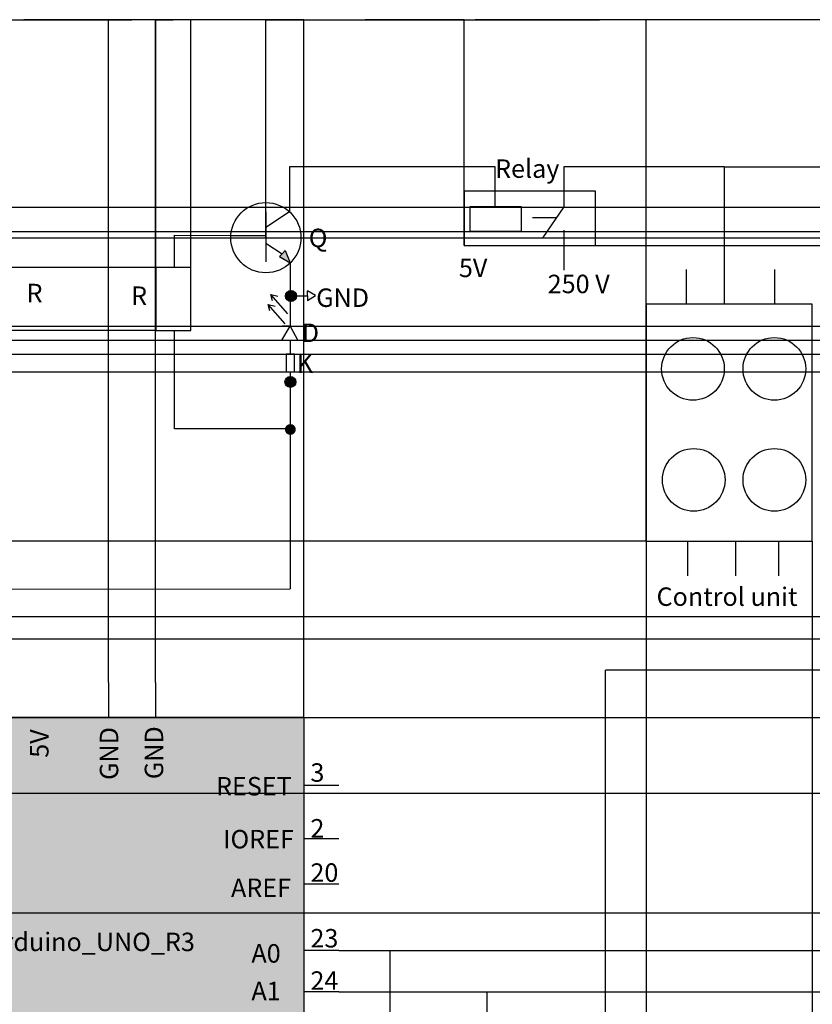
# Model space of a CAD drawing. Units: inches. Extents: x 35362 to 73946, y 43607 to 67532.
# Tile 134 of 134: x 57838 to 67327, y 55752 to 67532. Entities that reach past the tile are written whole.
import ezdxf

# ---------------------------------------------------------------- set-up
doc = ezdxf.new("R2010")
doc.units = ezdxf.units.IN
doc.header["$MEASUREMENT"] = 0
for name, color, linetype, lineweight in [('A-ANNO-DIMS', 2, 'Continuous', 18), ('E-ANNO-TEXT', 5, 'Continuous', 18), ('E-SYMB', 1, 'Continuous', 25), ('E-SYMB-PATT', 1, 'Continuous', 13), ('E-WIRE', 3, 'Continuous', 25)]:
    doc.layers.add(name, color=color, linetype=linetype, lineweight=lineweight)
doc.styles.get("Standard").update_dxf_attribs({"font": 'arial.ttf'})
doc.dimstyles.get("Standard").update_dxf_attribs({"dimtxt": 0.18, "dimasz": 0.18, "dimexe": 0.18, "dimexo": 0.0625, "dimgap": 0.09, "dimtad": 0, "dimtih": 1, "dimtoh": 1, "dimdec": 4, "dimzin": 0, "dimdsep": 46, "dimtxsty": 'Standard', "dimcen": 0.09, "dimadec": 0, "dimazin": 0, "dimtfac": 1, "dimtdec": 4, "dimtofl": 0, "dimtmove": 0, "dimatfit": 3, "dimfxl": 1, "dimtolj": 1, "dimtzin": 0, "dimarcsym": 0})

# ---------------------------------------------------------------- blocks, each defined once
blk = doc.blocks.new('*D8')
at = {"layer": 'A-ANNO-DIMS', "color": 0, "lineweight": -2, "transparency": 16777216}
for p, q in [((66271.28651900003, 65771.51172800003), (73945.82566600003, 65771.51172800003)), ((73945.64566600005, 65771.33172800003), (73945.64566600005, 59737.03093663782)), ((73945.64566600005, 53702.36633900002), (73945.64566600005, 59736.66713036224)), ((72185.70816600003, 53702.18633900003), (73945.82566600003, 53702.18633900003))]:
    blk.add_line(p, q, dxfattribs=at)
at = {"layer": 'A-ANNO-DIMS', "color": 0, "transparency": 16777216}
for points in [[(73945.61566600006, 65771.33172800003), (73945.67566600005, 65771.33172800003), (73945.64566600005, 65771.51172800003)], [(73945.61566600006, 53702.36633900002), (73945.67566600005, 53702.36633900002), (73945.64566600005, 53702.18633900003)]]:
    blk.add_solid(points, dxfattribs=at)
at = {"layer": 'Defpoints', "color": 0, "transparency": 16777216}
for p in [(66271.22401900003, 65771.51172800003), (73945.64566600005, 65771.51172800003), (72185.64566600003, 53702.18633900003)]:
    blk.add_point(p, dxfattribs=at)
at = {"layer": 'A-ANNO-DIMS', "color": 0, "transparency": 16777216, "insert": (73945.64566600005, 59736.84903349999), "char_height": 0.18, "attachment_point": 5}
blk.add_mtext('\\A1;12069', dxfattribs=at)
blk = doc.blocks.new('*D9')
at = {"layer": 'A-ANNO-DIMS', "color": 0, "lineweight": -2, "transparency": 16777216}
for p, q in [((56873.601939, 59185.206457), (56873.601939, 67531.691728)), ((56873.78193899999, 67531.51172799998), (59056.89224322987, 67531.51172799998)), ((61240.727336, 67531.51172799998), (59057.61703177011, 67531.51172799998)), ((61240.907336, 59185.206457), (61240.907336, 67531.691728))]:
    blk.add_line(p, q, dxfattribs=at)
at = {"layer": 'A-ANNO-DIMS', "color": 0, "transparency": 16777216}
for points in [[(56873.78193899999, 67531.541728), (56873.78193899999, 67531.481728), (56873.601939, 67531.51172799998)], [(61240.727336, 67531.541728), (61240.727336, 67531.481728), (61240.907336, 67531.51172799998)]]:
    blk.add_solid(points, dxfattribs=at)
at = {"layer": 'Defpoints', "color": 0, "transparency": 16777216}
for p in [(61240.907336, 67531.51172799998), (56873.601939, 59185.14395699999), (61240.907336, 59185.14395699999)]:
    blk.add_point(p, dxfattribs=at)
at = {"layer": 'A-ANNO-DIMS', "color": 0, "transparency": 16777216, "insert": (59057.25463749999, 67531.51172799998), "char_height": 0.18, "attachment_point": 5}
blk.add_mtext('\\A1;4367', dxfattribs=at)
blk = doc.blocks.new('*D10')
at = {"layer": 'A-ANNO-DIMS', "color": 0, "lineweight": -2, "transparency": 16777216}
for p, q in [((61240.96983600002, 59185.14395700003), (73945.82566600003, 59185.14395700003)), ((73945.64566600005, 59184.96395700003), (73945.64566600005, 56268.51827402935)), ((73945.64566600005, 53351.70866200003), (73945.64566600005, 56268.1543449707)), ((61240.96983600002, 53351.52866200003), (73945.82566600003, 53351.52866200003))]:
    blk.add_line(p, q, dxfattribs=at)
at = {"layer": 'A-ANNO-DIMS', "color": 0, "transparency": 16777216}
for points in [[(73945.61566600006, 59184.96395700003), (73945.67566600005, 59184.96395700003), (73945.64566600005, 59185.14395700003)], [(73945.61566600006, 53351.70866200003), (73945.67566600005, 53351.70866200003), (73945.64566600005, 53351.52866200003)]]:
    blk.add_solid(points, dxfattribs=at)
at = {"layer": 'Defpoints', "color": 0, "transparency": 16777216}
for p in [(61240.90733600002, 59185.14395700003), (61240.90733600002, 53351.52866200003), (73945.64566600005, 53351.52866200003)]:
    blk.add_point(p, dxfattribs=at)
at = {"layer": 'A-ANNO-DIMS', "color": 0, "transparency": 16777216, "insert": (73945.64566600005, 56268.33630949999), "char_height": 0.18, "attachment_point": 5}
blk.add_mtext('\\A1;5834', dxfattribs=at)
blk = doc.blocks.new('*D31')
at = {"layer": 'A-ANNO-DIMS', "color": 0, "lineweight": -2, "transparency": 16777216}
for p, q in [((56464.73443199999, 64923.81491999999), (56464.73443199999, 67531.69172799998)), ((56464.914432, 67531.51172799998), (58624.50560916985, 67531.51172799998)), ((60785.032639, 67531.51172799998), (58625.44146183015, 67531.51172799998)), ((60785.21263899999, 64923.81491999999), (60785.21263899999, 67531.69172799998))]:
    blk.add_line(p, q, dxfattribs=at)
at = {"layer": 'A-ANNO-DIMS', "color": 0, "transparency": 16777216}
for points in [[(56464.914432, 67531.541728), (56464.914432, 67531.481728), (56464.73443199999, 67531.51172799998)], [(60785.032639, 67531.541728), (60785.032639, 67531.481728), (60785.21263899999, 67531.51172799998)]]:
    blk.add_solid(points, dxfattribs=at)
at = {"layer": 'Defpoints', "color": 0, "transparency": 16777216}
for p in [(60785.21263899999, 67531.51172799998), (56464.73443199999, 64923.75241999999), (60785.21263899999, 64923.75241999999)]:
    blk.add_point(p, dxfattribs=at)
at = {"layer": 'A-ANNO-DIMS', "color": 0, "transparency": 16777216, "insert": (58624.9735355, 67531.51172799998), "char_height": 0.18, "attachment_point": 5}
blk.add_mtext('\\A1;4320.5', dxfattribs=at)
blk = doc.blocks.new('*D32')
at = {"layer": 'A-ANNO-DIMS', "color": 0, "lineweight": -2, "transparency": 16777216}
for p, q in [((60785.21263899999, 64923.81491999999), (60785.21263899999, 67531.69172799998)), ((60785.39263899999, 67531.51172799998), (61971.73112124693, 67531.51172799998)), ((63158.999317, 67531.51172799998), (61972.66083475307, 67531.51172799998)), ((63159.179317, 64828.618767), (63159.179317, 67531.69172799998))]:
    blk.add_line(p, q, dxfattribs=at)
at = {"layer": 'A-ANNO-DIMS', "color": 0, "transparency": 16777216}
for points in [[(60785.39263899999, 67531.541728), (60785.39263899999, 67531.481728), (60785.21263899999, 67531.51172799998)], [(63158.999317, 67531.541728), (63158.999317, 67531.481728), (63159.179317, 67531.51172799998)]]:
    blk.add_solid(points, dxfattribs=at)
at = {"layer": 'Defpoints', "color": 0, "transparency": 16777216}
for p in [(63159.179317, 67531.51172799998), (60785.21263899999, 64923.75241999999), (63159.179317, 64828.556267)]:
    blk.add_point(p, dxfattribs=at)
at = {"layer": 'A-ANNO-DIMS', "color": 0, "transparency": 16777216, "insert": (61972.195978, 67531.51172799998), "char_height": 0.18, "attachment_point": 5}
blk.add_mtext('\\A1;2374.0', dxfattribs=at)
blk = doc.blocks.new('*D33')
at = {"layer": 'A-ANNO-DIMS', "color": 0, "lineweight": -2, "transparency": 16777216}
for p, q in [((61240.907336, 59185.206457), (61240.907336, 67531.691728)), ((61241.08733599999, 67531.51172799998), (63288.01179478308, 67531.51172799998)), ((65335.836008, 67531.51172799998), (63288.91154921691, 67531.51172799998)), ((65336.01600799999, 61293.348552), (65336.01600799999, 67531.691728))]:
    blk.add_line(p, q, dxfattribs=at)
at = {"layer": 'A-ANNO-DIMS', "color": 0, "transparency": 16777216}
for points in [[(61241.08733599999, 67531.541728), (61241.08733599999, 67531.481728), (61240.907336, 67531.51172799998)], [(65335.836008, 67531.541728), (65335.836008, 67531.481728), (65336.01600799999, 67531.51172799998)]]:
    blk.add_solid(points, dxfattribs=at)
at = {"layer": 'Defpoints', "color": 0, "transparency": 16777216}
for p in [(65336.01600799999, 67531.51172799998), (65336.01600799999, 61293.286052), (61240.907336, 59185.14395699999)]:
    blk.add_point(p, dxfattribs=at)
at = {"layer": 'A-ANNO-DIMS', "color": 0, "transparency": 16777216, "insert": (63288.461672, 67531.51172799998), "char_height": 0.18, "attachment_point": 5}
blk.add_mtext('\\A1;4095.1', dxfattribs=at)
blk = doc.blocks.new('*D34')
at = {"layer": 'A-ANNO-DIMS', "color": 0, "lineweight": -2, "transparency": 16777216}
for p, q in [((65335.95350800003, 61293.28605200003), (35361.76908500003, 61293.28605200003)), ((35361.94908500003, 61293.10605200002), (35361.94908500003, 60239.39690763781)), ((35361.94908500003, 59185.32395700002), (35361.94908500003, 60239.03310136224)), ((61240.84483600002, 59185.14395700003), (35361.76908500003, 59185.14395700002))]:
    blk.add_line(p, q, dxfattribs=at)
at = {"layer": 'A-ANNO-DIMS', "color": 0, "transparency": 16777216}
for points in [[(35361.91908500003, 61293.10605200002), (35361.97908500003, 61293.10605200002), (35361.94908500003, 61293.28605200003)], [(35361.91908500003, 59185.32395700002), (35361.97908500003, 59185.32395700002), (35361.94908500003, 59185.14395700002)]]:
    blk.add_solid(points, dxfattribs=at)
at = {"layer": 'Defpoints', "color": 0, "transparency": 16777216}
for p in [(65336.01600800003, 61293.28605200003), (35361.94908500003, 59185.14395700002), (61240.90733600002, 59185.14395700003)]:
    blk.add_point(p, dxfattribs=at)
at = {"layer": 'A-ANNO-DIMS', "color": 0, "transparency": 16777216, "insert": (35361.94908500005, 60239.2150045), "char_height": 0.18, "attachment_point": 5}
blk.add_mtext('\\A1;2108.1', dxfattribs=at)
blk = doc.blocks.new('*D35')
at = {"layer": 'A-ANNO-DIMS', "color": 0, "lineweight": -2, "transparency": 16777216}
for p, q in [((61240.907336, 59185.206457), (61240.907336, 67531.691728)), ((61241.08733599999, 67531.51172799998), (64780.42646373397, 67531.51172799998)), ((68320.69076200001, 67531.51172799998), (64781.35163426603, 67531.51172799998)), ((68320.870762, 60122.408832), (68320.870762, 67531.691728))]:
    blk.add_line(p, q, dxfattribs=at)
at = {"layer": 'A-ANNO-DIMS', "color": 0, "transparency": 16777216}
for points in [[(61241.08733599999, 67531.541728), (61241.08733599999, 67531.481728), (61240.907336, 67531.51172799998)], [(68320.69076200001, 67531.541728), (68320.69076200001, 67531.481728), (68320.870762, 67531.51172799998)]]:
    blk.add_solid(points, dxfattribs=at)
at = {"layer": 'Defpoints', "color": 0, "transparency": 16777216}
for p in [(68320.870762, 67531.51172799998), (68320.870762, 60122.346332), (61240.907336, 59185.14395699999)]:
    blk.add_point(p, dxfattribs=at)
at = {"layer": 'A-ANNO-DIMS', "color": 0, "transparency": 16777216, "insert": (64780.889049, 67531.51172799998), "char_height": 0.18, "attachment_point": 5}
blk.add_mtext('\\A1;7080.0', dxfattribs=at)
blk = doc.blocks.new('*D36')
at = {"layer": 'A-ANNO-DIMS', "color": 0, "lineweight": -2, "transparency": 16777216}
for p, q in [((68320.80826200004, 60122.34633200002), (35361.76908500003, 60122.34633200002)), ((35361.94908500003, 60122.16633200002), (35361.94908500003, 57247.82893113781)), ((35361.94908500003, 54373.12772400002), (35361.94908500003, 57247.46512486223)), ((68320.80826200004, 54372.94772400003), (35361.76908500003, 54372.94772400002))]:
    blk.add_line(p, q, dxfattribs=at)
at = {"layer": 'A-ANNO-DIMS', "color": 0, "transparency": 16777216}
for points in [[(35361.91908500003, 60122.16633200002), (35361.97908500003, 60122.16633200002), (35361.94908500003, 60122.34633200002)], [(35361.91908500003, 54373.12772400002), (35361.97908500003, 54373.12772400002), (35361.94908500003, 54372.94772400002)]]:
    blk.add_solid(points, dxfattribs=at)
at = {"layer": 'Defpoints', "color": 0, "transparency": 16777216}
for p in [(68320.87076200004, 60122.34633200002), (35361.94908500003, 54372.94772400002), (68320.87076200004, 54372.94772400003)]:
    blk.add_point(p, dxfattribs=at)
at = {"layer": 'A-ANNO-DIMS', "color": 0, "transparency": 16777216, "insert": (35361.94908500004, 57247.64702799999), "char_height": 0.18, "attachment_point": 5}
blk.add_mtext('\\A1;5749.4', dxfattribs=at)
blk = doc.blocks.new('*D47')
at = {"layer": 'A-ANNO-DIMS', "color": 0, "lineweight": -2, "transparency": 16777216}
for p, q in [((50339.58680000003, 58279.98849500002), (73945.82566600003, 58279.98849500002)), ((73945.64566600005, 58279.80849500002), (73945.64566600005, 57564.17141502935)), ((73945.64566600005, 56848.17040600003), (73945.64566600005, 57563.80748597069)), ((50339.58680000003, 56847.99040600003), (73945.82566600003, 56847.99040600003))]:
    blk.add_line(p, q, dxfattribs=at)
at = {"layer": 'A-ANNO-DIMS', "color": 0, "transparency": 16777216}
for points in [[(73945.61566600006, 58279.80849500002), (73945.67566600005, 58279.80849500002), (73945.64566600005, 58279.98849500002)], [(73945.61566600006, 56848.17040600003), (73945.67566600005, 56848.17040600003), (73945.64566600005, 56847.99040600003)]]:
    blk.add_solid(points, dxfattribs=at)
at = {"layer": 'Defpoints', "color": 0, "transparency": 16777216}
for p in [(50339.52430000002, 58279.98849500002), (50339.52430000002, 56847.99040600003), (73945.64566600005, 56847.99040600003)]:
    blk.add_point(p, dxfattribs=at)
at = {"layer": 'A-ANNO-DIMS', "color": 0, "transparency": 16777216, "insert": (73945.64566600005, 57563.98945049999), "char_height": 0.18, "attachment_point": 5}
blk.add_mtext('\\A1;1432.0', dxfattribs=at)
blk = doc.blocks.new('*D50')
at = {"layer": 'A-ANNO-DIMS', "color": 0, "lineweight": -2, "transparency": 16777216}
for p, q in [((61657.28213900003, 56394.41825000003), (73945.82566600003, 56394.41825000003)), ((73945.64566600005, 56394.23825000003), (73945.64566600005, 56147.19337413782)), ((73945.64566600005, 55899.78469200003), (73945.64566600005, 56146.82956786224)), ((61657.28213900003, 55899.60469200002), (73945.82566600003, 55899.60469200002))]:
    blk.add_line(p, q, dxfattribs=at)
at = {"layer": 'A-ANNO-DIMS', "color": 0, "transparency": 16777216}
for points in [[(73945.61566600006, 56394.23825000003), (73945.67566600005, 56394.23825000003), (73945.64566600005, 56394.41825000003)], [(73945.61566600006, 55899.78469200003), (73945.67566600005, 55899.78469200003), (73945.64566600005, 55899.60469200002)]]:
    blk.add_solid(points, dxfattribs=at)
at = {"layer": 'Defpoints', "color": 0, "transparency": 16777216}
for p in [(61657.21963900003, 56394.41825000003), (61657.21963900003, 55899.60469200002), (73945.64566600005, 55899.60469200002)]:
    blk.add_point(p, dxfattribs=at)
at = {"layer": 'A-ANNO-DIMS', "color": 0, "transparency": 16777216, "insert": (73945.64566600005, 56147.01147099999), "char_height": 0.18, "attachment_point": 5}
blk.add_mtext('\\A1;494.8', dxfattribs=at)
blk = doc.blocks.new('*D51')
at = {"layer": 'A-ANNO-DIMS', "color": 0, "lineweight": -2, "transparency": 16777216}
for p, q in [((56873.601939, 59185.206457), (56873.601939, 67531.691728)), ((56873.78193899999, 67531.51172799998), (57886.0318306146, 67531.51172799998)), ((58899.212418, 67531.51172799998), (57886.9625263854, 67531.51172799998)), ((58899.392418, 59601.518759), (58899.392418, 67531.691728))]:
    blk.add_line(p, q, dxfattribs=at)
at = {"layer": 'A-ANNO-DIMS', "color": 0, "transparency": 16777216}
for points in [[(56873.78193899999, 67531.541728), (56873.78193899999, 67531.481728), (56873.601939, 67531.51172799998)], [(58899.212418, 67531.541728), (58899.212418, 67531.481728), (58899.392418, 67531.51172799998)]]:
    blk.add_solid(points, dxfattribs=at)
at = {"layer": 'Defpoints', "color": 0, "transparency": 16777216}
for p in [(58899.392418, 67531.51172799998), (58899.392418, 59601.456259), (56873.601939, 59185.14395699999)]:
    blk.add_point(p, dxfattribs=at)
at = {"layer": 'A-ANNO-DIMS', "color": 0, "transparency": 16777216, "insert": (57886.4971785, 67531.51172799998), "char_height": 0.18, "attachment_point": 5}
blk.add_mtext('\\A1;2025.8', dxfattribs=at)
blk = doc.blocks.new('*D52')
at = {"layer": 'A-ANNO-DIMS', "color": 0, "lineweight": -2, "transparency": 16777216}
for p, q in [((58899.392418, 59601.518759), (58899.392418, 67531.691728)), ((58899.572418, 67531.51172799998), (59181.94888036904, 67531.51172799998)), ((59465.113119, 67531.51172799998), (59182.73665663097, 67531.51172799998)), ((59465.293119, 59601.518759), (59465.293119, 67531.691728))]:
    blk.add_line(p, q, dxfattribs=at)
at = {"layer": 'A-ANNO-DIMS', "color": 0, "transparency": 16777216}
for points in [[(58899.572418, 67531.541728), (58899.572418, 67531.481728), (58899.392418, 67531.51172799998)], [(59465.113119, 67531.541728), (59465.113119, 67531.481728), (59465.293119, 67531.51172799998)]]:
    blk.add_solid(points, dxfattribs=at)
at = {"layer": 'Defpoints', "color": 0, "transparency": 16777216}
for p in [(59465.293119, 67531.51172799998), (58899.392418, 59601.456259), (59465.293119, 59601.456259)]:
    blk.add_point(p, dxfattribs=at)
at = {"layer": 'A-ANNO-DIMS', "color": 0, "transparency": 16777216, "insert": (59182.3427685, 67531.51172799998), "char_height": 0.18, "attachment_point": 5}
blk.add_mtext('\\A1;565.9', dxfattribs=at)
blk = doc.blocks.new('*D65')
at = {"layer": 'A-ANNO-DIMS', "color": 0, "lineweight": -2, "transparency": 16777216}
for p, q in [((65336.01600799999, 61293.223552), (65336.01600799999, 43606.678996)), ((67326.639741, 61293.223552), (67326.639741, 43606.678996)), ((65336.19600799999, 43606.858996), (66330.87277900206, 43606.858996)), ((67326.45974100001, 43606.858996), (66331.78296999796, 43606.858996))]:
    blk.add_line(p, q, dxfattribs=at)
at = {"layer": 'A-ANNO-DIMS', "color": 0, "transparency": 16777216}
for points in [[(65336.19600799999, 43606.888996), (65336.19600799999, 43606.828996), (65336.01600799999, 43606.858996)], [(67326.45974100001, 43606.888996), (67326.45974100001, 43606.828996), (67326.639741, 43606.858996)]]:
    blk.add_solid(points, dxfattribs=at)
at = {"layer": 'Defpoints', "color": 0, "transparency": 16777216}
for p in [(65336.01600799999, 61293.286052), (67326.639741, 61293.286052), (67326.639741, 43606.858996)]:
    blk.add_point(p, dxfattribs=at)
at = {"layer": 'A-ANNO-DIMS', "color": 0, "transparency": 16777216, "insert": (66331.32787450001, 43606.858996), "char_height": 0.18, "attachment_point": 5}
blk.add_mtext('\\A1;1990.6', dxfattribs=at)
blk = doc.blocks.new('*D70')
at = {"layer": 'A-ANNO-DIMS', "color": 0, "lineweight": -2, "transparency": 16777216}
for p, q in [((60785.27513900002, 64923.75242000003), (73945.82566600003, 64923.75242000003)), ((73945.64566600005, 64923.57242000003), (73945.64566600005, 62054.63015302935)), ((73945.64566600005, 59185.32395700003), (73945.64566600005, 62054.26622397069)), ((61240.96983600002, 59185.14395700003), (73945.82566600003, 59185.14395700003))]:
    blk.add_line(p, q, dxfattribs=at)
at = {"layer": 'A-ANNO-DIMS', "color": 0, "transparency": 16777216}
for points in [[(73945.61566600006, 64923.57242000003), (73945.67566600005, 64923.57242000003), (73945.64566600005, 64923.75242000003)], [(73945.61566600006, 59185.32395700003), (73945.67566600005, 59185.32395700003), (73945.64566600005, 59185.14395700003)]]:
    blk.add_solid(points, dxfattribs=at)
at = {"layer": 'Defpoints', "color": 0, "transparency": 16777216}
for p in [(60785.21263900002, 64923.75242000003), (73945.64566600005, 64923.75242000003), (61240.90733600002, 59185.14395700003)]:
    blk.add_point(p, dxfattribs=at)
at = {"layer": 'A-ANNO-DIMS', "color": 0, "transparency": 16777216, "insert": (73945.64566600005, 62054.44818849999), "char_height": 0.18, "attachment_point": 5}
blk.add_mtext('\\A1;5738.6', dxfattribs=at)
blk = doc.blocks.new('*D71')
at = {"layer": 'A-ANNO-DIMS', "color": 0, "lineweight": -2, "transparency": 16777216}
for p, q in [((63159.24181700003, 64828.55626700002), (73945.82566600003, 64828.55626700002)), ((73945.64566600005, 64828.37626700002), (73945.64566600005, 62007.03207652936)), ((73945.64566600005, 59185.32395700003), (73945.64566600005, 62006.6681474707)), ((61240.96983600002, 59185.14395700003), (73945.82566600003, 59185.14395700003))]:
    blk.add_line(p, q, dxfattribs=at)
at = {"layer": 'A-ANNO-DIMS', "color": 0, "transparency": 16777216}
for points in [[(73945.61566600006, 64828.37626700002), (73945.67566600005, 64828.37626700002), (73945.64566600005, 64828.55626700002)], [(73945.61566600006, 59185.32395700003), (73945.67566600005, 59185.32395700003), (73945.64566600005, 59185.14395700003)]]:
    blk.add_solid(points, dxfattribs=at)
at = {"layer": 'Defpoints', "color": 0, "transparency": 16777216}
for p in [(63159.17931700003, 64828.55626700002), (73945.64566600005, 64828.55626700002), (61240.90733600002, 59185.14395700003)]:
    blk.add_point(p, dxfattribs=at)
at = {"layer": 'A-ANNO-DIMS', "color": 0, "transparency": 16777216, "insert": (73945.64566600005, 62006.85011199999), "char_height": 0.18, "attachment_point": 5}
blk.add_mtext('\\A1;5643.4', dxfattribs=at)
blk = doc.blocks.new('*D72')
at = {"layer": 'A-ANNO-DIMS', "color": 0, "lineweight": -2, "transparency": 16777216}
for p, q in [((59468.795591, 64568.03448599999), (59468.795591, 67531.69172799998)), ((59468.975591, 67531.51172799998), (59676.86363976808, 67531.51172799998)), ((59885.546709, 67531.51172799998), (59677.65866023193, 67531.51172799998)), ((59885.726709, 64568.03448599999), (59885.726709, 67531.69172799998))]:
    blk.add_line(p, q, dxfattribs=at)
at = {"layer": 'A-ANNO-DIMS', "color": 0, "transparency": 16777216}
for points in [[(59468.975591, 67531.541728), (59468.975591, 67531.481728), (59468.795591, 67531.51172799998)], [(59885.546709, 67531.541728), (59885.546709, 67531.481728), (59885.726709, 67531.51172799998)]]:
    blk.add_solid(points, dxfattribs=at)
at = {"layer": 'Defpoints', "color": 0, "transparency": 16777216}
for p in [(59885.726709, 67531.51172799998), (59468.795591, 64567.971986), (59885.726709, 64567.971986)]:
    blk.add_point(p, dxfattribs=at)
at = {"layer": 'A-ANNO-DIMS', "color": 0, "transparency": 16777216, "insert": (59677.26115, 67531.51172799998), "char_height": 0.18, "attachment_point": 5}
blk.add_mtext('\\A1;416.9', dxfattribs=at)
blk = doc.blocks.new('*D73')
at = {"layer": 'A-ANNO-DIMS', "color": 0, "lineweight": -2, "transparency": 16777216}
for p, q in [((59468.73309100003, 64567.97198600003), (35361.76908500003, 64567.97198600002)), ((35361.94908500003, 64567.79198600002), (35361.94908500003, 64189.84474213781)), ((35361.94908500003, 63811.53369200002), (35361.94908500003, 64189.48093586223)), ((59468.73309100003, 63811.35369200002), (35361.76908500003, 63811.35369200002))]:
    blk.add_line(p, q, dxfattribs=at)
at = {"layer": 'A-ANNO-DIMS', "color": 0, "transparency": 16777216}
for points in [[(35361.91908500003, 64567.79198600002), (35361.97908500003, 64567.79198600002), (35361.94908500003, 64567.97198600002)], [(35361.91908500003, 63811.53369200002), (35361.97908500003, 63811.53369200002), (35361.94908500003, 63811.35369200002)]]:
    blk.add_solid(points, dxfattribs=at)
at = {"layer": 'Defpoints', "color": 0, "transparency": 16777216}
for p in [(35361.94908500003, 64567.97198600002), (59468.79559100003, 64567.97198600003), (59468.79559100003, 63811.35369200002)]:
    blk.add_point(p, dxfattribs=at)
at = {"layer": 'A-ANNO-DIMS', "color": 0, "transparency": 16777216, "insert": (35361.94908500005, 64189.66283899999), "char_height": 0.18, "attachment_point": 5}
blk.add_mtext('\\A1;756.6', dxfattribs=at)
blk = doc.blocks.new('*D97')
at = {"layer": 'A-ANNO-DIMS', "color": 0, "lineweight": -2, "transparency": 16777216}
for p, q in [((53988.67814800002, 65288.88854300003), (73945.82566600003, 65288.88854300003)), ((73945.64566600005, 65288.70854300003), (73945.64566600005, 65143.46751513782)), ((73945.64566600005, 64997.86268100002), (73945.64566600005, 65143.10370886223)), ((53988.67814800002, 64997.68268100003), (73945.82566600003, 64997.68268100003))]:
    blk.add_line(p, q, dxfattribs=at)
at = {"layer": 'A-ANNO-DIMS', "color": 0, "transparency": 16777216}
for points in [[(73945.61566600006, 65288.70854300003), (73945.67566600005, 65288.70854300003), (73945.64566600005, 65288.88854300003)], [(73945.61566600006, 64997.86268100002), (73945.67566600005, 64997.86268100002), (73945.64566600005, 64997.68268100003)]]:
    blk.add_solid(points, dxfattribs=at)
at = {"layer": 'Defpoints', "color": 0, "transparency": 16777216}
for p in [(53988.61564800003, 65288.88854300003), (73945.64566600005, 65288.88854300003), (53988.61564800003, 64997.68268100003)]:
    blk.add_point(p, dxfattribs=at)
at = {"layer": 'A-ANNO-DIMS', "color": 0, "transparency": 16777216, "insert": (73945.64566600005, 65143.28561199999), "char_height": 0.18, "attachment_point": 5}
blk.add_mtext('\\A1;291.2', dxfattribs=at)
blk = doc.blocks.new('*D103')
at = {"layer": 'A-ANNO-DIMS', "color": 0, "lineweight": -2, "transparency": 16777216}
for p, q in [((56172.14479300002, 63863.49026700003), (73945.82566600003, 63863.49026700003)), ((73945.64566600005, 63863.31026700003), (73945.64566600005, 63780.36050313782)), ((73945.64566600005, 63697.04693300002), (73945.64566600005, 63779.99669686224)), ((56272.53121400003, 63696.86693300002), (73945.82566600003, 63696.86693300002))]:
    blk.add_line(p, q, dxfattribs=at)
at = {"layer": 'A-ANNO-DIMS', "color": 0, "transparency": 16777216}
for points in [[(73945.61566600006, 63863.31026700003), (73945.67566600005, 63863.31026700003), (73945.64566600005, 63863.49026700003)], [(73945.61566600006, 63697.04693300002), (73945.67566600005, 63697.04693300002), (73945.64566600005, 63696.86693300002)]]:
    blk.add_solid(points, dxfattribs=at)
at = {"layer": 'Defpoints', "color": 0, "transparency": 16777216}
for p in [(56172.08229300002, 63863.49026700003), (73945.64566600005, 63863.49026700003), (56272.46871400003, 63696.86693300002)]:
    blk.add_point(p, dxfattribs=at)
at = {"layer": 'A-ANNO-DIMS', "color": 0, "transparency": 16777216, "insert": (73945.64566600005, 63780.17859999999), "char_height": 0.18, "attachment_point": 5}
blk.add_mtext('\\A1;166.62', dxfattribs=at)
blk = doc.blocks.new('*D105')
at = {"layer": 'A-ANNO-DIMS', "color": 0, "lineweight": -2, "transparency": 16777216}
for p, q in [((56223.01523600002, 63531.49645700002), (73945.82566600003, 63531.49645700002)), ((73945.64566600005, 63531.31645700003), (73945.64566600005, 63424.99614102936)), ((73945.64566600005, 63318.31189600003), (73945.64566600005, 63424.6322119707)), ((56223.01523600002, 63318.13189600002), (73945.82566600003, 63318.13189600002))]:
    blk.add_line(p, q, dxfattribs=at)
at = {"layer": 'A-ANNO-DIMS', "color": 0, "transparency": 16777216}
for points in [[(73945.61566600006, 63531.31645700003), (73945.67566600005, 63531.31645700003), (73945.64566600005, 63531.49645700002)], [(73945.61566600006, 63318.31189600003), (73945.67566600005, 63318.31189600003), (73945.64566600005, 63318.13189600002)]]:
    blk.add_solid(points, dxfattribs=at)
at = {"layer": 'Defpoints', "color": 0, "transparency": 16777216}
for p in [(56222.95273600003, 63531.49645700002), (73945.64566600005, 63531.49645700002), (56222.95273600003, 63318.13189600002)]:
    blk.add_point(p, dxfattribs=at)
at = {"layer": 'A-ANNO-DIMS', "color": 0, "transparency": 16777216, "insert": (73945.64566600005, 63424.8141765), "char_height": 0.18, "attachment_point": 5}
blk.add_mtext('\\A1;213.36', dxfattribs=at)
blk = doc.blocks.new('*D106')
at = {"layer": 'A-ANNO-DIMS', "color": 0, "lineweight": -2, "transparency": 16777216}
for p, q in [((56464.79693200002, 64923.75242000003), (73945.82566600003, 64923.75242000003)), ((73945.64566600005, 64923.57242000003), (73945.64566600005, 64393.80330802936)), ((73945.64566600005, 63863.67026700003), (73945.64566600005, 64393.4393789707)), ((56172.14479300002, 63863.49026700003), (73945.82566600003, 63863.49026700003))]:
    blk.add_line(p, q, dxfattribs=at)
at = {"layer": 'A-ANNO-DIMS', "color": 0, "transparency": 16777216}
for points in [[(73945.61566600006, 64923.57242000003), (73945.67566600005, 64923.57242000003), (73945.64566600005, 64923.75242000003)], [(73945.61566600006, 63863.67026700003), (73945.67566600005, 63863.67026700003), (73945.64566600005, 63863.49026700003)]]:
    blk.add_solid(points, dxfattribs=at)
at = {"layer": 'Defpoints', "color": 0, "transparency": 16777216}
for p in [(56464.73443200003, 64923.75242000003), (56172.08229300002, 63863.49026700003), (73945.64566600005, 63863.49026700003)]:
    blk.add_point(p, dxfattribs=at)
at = {"layer": 'A-ANNO-DIMS', "color": 0, "transparency": 16777216, "insert": (73945.64566600005, 64393.62134349998), "char_height": 0.18, "attachment_point": 5}
blk.add_mtext('\\A1;1060.3', dxfattribs=at)
blk = doc.blocks.new('*D113')
at = {"layer": 'A-ANNO-DIMS', "color": 0, "lineweight": -2, "transparency": 16777216}
for p, q in [((53526.13474100003, 60391.71935800003), (73945.82566600003, 60391.71935800003)), ((73945.64566600005, 60391.53935800003), (73945.64566600005, 60259.19182863781)), ((73945.64566600005, 60126.48049300003), (73945.64566600005, 60258.82802236224)), ((53705.42262200003, 60126.30049300003), (73945.82566600003, 60126.30049300003))]:
    blk.add_line(p, q, dxfattribs=at)
at = {"layer": 'A-ANNO-DIMS', "color": 0, "transparency": 16777216}
for points in [[(73945.61566600006, 60391.53935800003), (73945.67566600005, 60391.53935800003), (73945.64566600005, 60391.71935800003)], [(73945.61566600006, 60126.48049300003), (73945.67566600005, 60126.48049300003), (73945.64566600005, 60126.30049300003)]]:
    blk.add_solid(points, dxfattribs=at)
at = {"layer": 'Defpoints', "color": 0, "transparency": 16777216}
for p in [(53526.07224100003, 60391.71935800003), (73945.64566600005, 60391.71935800003), (53705.36012200003, 60126.30049300003)]:
    blk.add_point(p, dxfattribs=at)
at = {"layer": 'A-ANNO-DIMS', "color": 0, "transparency": 16777216, "insert": (73945.64566600005, 60259.00992549999), "char_height": 0.18, "attachment_point": 5}
blk.add_mtext('\\A1;265.4', dxfattribs=at)

msp = doc.modelspace()

# ---------------------------------------------------------------- hatches: boundary and pattern name
at = {"layer": 'E-SYMB-PATT'}
h = msp.add_hatch(color=256, dxfattribs=at)
h.dxf.hatch_style = 1
h.paths.add_polyline_path([(61077.86477877302, 64622.77542694354), (60947.29952449183, 64696.96561866228), (60981.59798827711, 64732.45736103127), (61017.73479179456, 64769.8514008492)])
h = msp.add_hatch(color=256, dxfattribs=at)
h.dxf.hatch_style = 1
h.paths.add_polyline_path([(61086.0385085762, 64291.02080926311, -0.4142135623730951), (61151.24345952185, 64225.81585831745, -0.4142135623730951), (61086.0385085762, 64160.61090737181)])
h.paths.add_polyline_path([(61086.0385085762, 64291.02080926311), (61086.0385085762, 64160.61090737181, -0.4142135623730951), (61020.83355763054, 64225.81585831745, -0.4142135623730951)])
h = msp.add_hatch(color=256, dxfattribs=at)
h.dxf.hatch_style = 1
h.paths.add_polyline_path([(61078.29748026865, 63262.79926251772, -0.4142135623730951), (61143.5024312143, 63197.59431157207, -0.4142135623730951), (61078.29748026865, 63132.38936062642)])
h.paths.add_polyline_path([(61078.29748026865, 63262.79926251772), (61078.29748026865, 63132.38936062642, -0.4142135623730951), (61013.09252932298, 63197.59431157207, -0.4142135623730951)])
h = msp.add_hatch(color=256, dxfattribs=at)
h.dxf.hatch_style = 1
h.paths.add_polyline_path([(61078.29748026865, 62694.1542046065, -0.4142135623730951), (61143.5024312143, 62628.94925366084, -0.4142135623730951), (61078.29748026865, 62563.7443027152)])
h.paths.add_polyline_path([(61078.29748026865, 62694.1542046065), (61078.29748026865, 62563.7443027152, -0.4142135623730951), (61013.09252932298, 62628.94925366084, -0.4142135623730951)])
h = msp.add_hatch(color=256, dxfattribs=at)
h.dxf.hatch_style = 1
h.paths.add_polyline_path([(56873.60193850077, 59185.14395657572), (56873.60193850077, 53351.5286622623), (61240.90733594325, 53351.5286622623), (61240.90733594325, 59185.14395657572)])

# ---------------------------------------------------------------- linework, layer by layer
at = {"layer": 'E-SYMB'}
for p, q in [((63528.44199587452, 65446.35464764817), (63528.44199587452, 65771.51172838474)), ((66271.22401929351, 65771.51172838474), (64352.46682501879, 65771.51172838474)), ((64352.46682501879, 65771.51172838474), (64352.46682501879, 65446.35464764817)), ((61066.57479254919, 65390.54203668585), (61066.57479254919, 65234.62536998068)), ((63528.44199587452, 65291.58881705664), (63528.44199587452, 65446.35464764817)), ((64352.46682501879, 65446.35464764817), (64352.46682501879, 65291.58881705664)), ((64352.46682501879, 65291.58881705664), (64099.28527020179, 64926.13796197845)), ((60785.21263932547, 65234.62536998068), (60785.21263932547, 64749.5524176359)), ((61066.57479254919, 65234.62536998068), (60785.21263932547, 65045.79413245495)), ((64261.24883334924, 65159.9216698261), (63975.18756389523, 65159.31277594798)), ((60366.34913702609, 64951.78438723841), (60785.21263932547, 64947.86055117672)), ((64352.46682501879, 65011.85664056519), (64352.46682501879, 64533.20102869082)), ((60785.21263932547, 64859.40556100751), (60981.59798827711, 64732.45736103127)), ((60785.21263932547, 64749.5524176359), (60785.21263932547, 64633.38684027922)), ((60981.59798827711, 64732.45736103127), (60947.29952449183, 64696.96561866228)), ((60947.29952449183, 64696.96561866228), (61077.86477877302, 64622.77542694354)), ((60981.59798827711, 64732.45736103127), (61017.73479179456, 64769.8514008492)), ((61017.73479179456, 64769.8514008492), (61077.86477877302, 64622.77542694354)), ((61077.86477877302, 64622.77542694354), (61077.86477877302, 64398.46363840721)), ((65816.73692390183, 64543.75391069253), (65816.73692390183, 64127.44160804251)), ((66873.18213873729, 64543.75391069253), (66873.18213873729, 64127.44160804251)), ((61047.24582755026, 64012.64072569341), (60844.76142281076, 64242.76765250924)), ((60844.76142281076, 64242.76765250924), (60928.95625311504, 64223.13849935204)), ((60862.63890963921, 64167.6760520751), (60844.76142281076, 64242.76765250924)), ((61151.17391143479, 64228.82665925307), (61284.72394970569, 64228.82665925307)), ((61284.72394970569, 64228.82665925307), (61284.72394970569, 64285.87207165673)), ((61380.8809793974, 64233.18598564114), (61284.72394970569, 64285.87207165673)), ((61284.72394970569, 64171.7812468494), (61380.8809793974, 64233.18598564114)), ((61284.72394970569, 64228.82665925307), (61284.72394970569, 64171.7812468494)), ((61015.41333267972, 63892.33325232277), (60812.92892794021, 64122.46017913862)), ((60812.92892794021, 64122.46017913862), (60897.1237582445, 64102.83102598142)), ((60830.80641476867, 64047.36857870447), (60812.92892794021, 64122.46017913862)), ((61077.86477877302, 64072.74030102532), (61077.86477877302, 63863.4902670446)), ((60977.47835771379, 63696.86693335817), (61077.86477877302, 63863.4902670446)), ((61077.86477877302, 63863.4902670446), (60984.06497884552, 63863.4902670446)), ((61077.86477877302, 63863.4902670446), (61171.66457870052, 63863.4902670446)), ((61077.86477877302, 63863.4902670446), (61169.45862435619, 63694.75541966131)), ((61169.45862435619, 63694.75541966131), (60977.47835771379, 63696.86693335817)), ((61077.86477877301, 63695.76282351005), (61077.86477877302, 63531.49645690672)), ((61077.86477877302, 63318.13189576597), (61077.86477877302, 63247.06648261227)), ((65831.62155391974, 61293.28605165897), (65831.62155391974, 60876.97374900895)), ((66407.91823292105, 61293.28605165897), (66407.91823292105, 60876.97374900895)), ((66920.07966787461, 61293.28605165897), (66920.07966787461, 60876.97374900895)), ((58899.39241832076, 59601.45625922574), (58899.39241832076, 59185.14395657572)), ((59465.29311933312, 59601.45625922574), (59465.29311933312, 59185.14395657572)), ((61657.21963859326, 58371.04947149105), (61240.90733594325, 58371.04947149105)), ((61657.21963859326, 57732.02855824052), (61240.90733594325, 57732.02855824052)), ((61657.21963859326, 57188.62445833935), (61240.90733594325, 57188.62445833935)), ((61657.21963859326, 56394.41825037897), (61240.90733594325, 56394.41825037897)), ((61657.21963859326, 55899.6046918906), (61240.90733594325, 55899.6046918906))]:
    msp.add_line(p, q, dxfattribs=at)
for points in [[(64732.14929761097, 65478.87035572184), (63159.17931741086, 65478.87035572184), (63159.17931741086, 64828.55626680058), (64732.14929761097, 64828.55626680058)], [(63846.70878040936, 65291.58881705664), (63224.8588657272, 65291.58881705664), (63224.8588657272, 65000.38295531353), (63846.70878040936, 65000.38295531353)], [(59885.72670946524, 64567.97198591175), (59468.79559058535, 64567.97198591175), (59468.79559058535, 63811.353692237), (59885.72670946524, 63811.353692237)], [(67326.63974086114, 64127.44160804251), (65336.01600767068, 64127.44160804251), (65336.01600767068, 61293.28605165897), (67326.63974086114, 61293.28605165897)], [(61126.73414854594, 63531.49645690672), (61026.99433572995, 63531.49645690672), (61026.99433572995, 63318.13189576597), (61126.73414854594, 63318.13189576597)], [(56873.60193850077, 59185.14395657572), (61240.90733594325, 59185.14395657572), (61240.90733594325, 53351.5286622623), (56873.60193850077, 53351.5286622623)]]:
    msp.add_lwpolyline(points, close=True, dxfattribs=at)
for centre, radius in [((60785.21263932547, 64923.75241950339), 419.8004582817891), ((61086.0385085762, 64225.81585831748), 65.20495094565227), ((65898.03235981136, 63354.17630024896), 375.1267449472869), ((66872.18743286145, 63354.17630024896), 375.1267449472869), ((61078.29748026865, 63197.59431157208), 65.20495094565227), ((65907.06181993964, 62026.02454863995), 375.1267449472869), ((66872.18743286145, 62026.02454863995), 375.1267449472869)]:
    msp.add_circle(centre, radius, dxfattribs=at)
at = {"layer": 'E-WIRE'}
for p, q in [((63528.44199587453, 65771.51172838474), (61066.57479254919, 65771.51172838474)), ((61066.57479254919, 65771.51172838474), (61066.57479254919, 65390.54203668585)), ((66271.22401929351, 65771.51172838474), (66271.22401929351, 64127.44160804251)), ((59690.02486826518, 64567.97198591175), (59690.02486826518, 64952.32836962721)), ((59690.02486826518, 64952.32836962721), (60366.34913702609, 64951.78438723841)), ((61077.86477877302, 64398.46363840721), (61077.86477877302, 64072.74030102532)), ((59690.02486826518, 62638.17010037096), (59690.02486826518, 63811.353692237)), ((61077.86477877302, 63247.06648261227), (61077.86477877302, 61661.75847953682)), ((61077.86477877302, 62638.17010037096), (59690.02486826518, 62638.17010037096)), ((61077.86477877302, 61661.75847953682), (61077.86477877302, 60722.33878634466)), ((55796.17232646729, 60718.22759180931), (61077.86477877302, 60722.33878634466)), ((64849.63466818351, 54587.23758632809), (64849.6346681835, 59750.68874003685)), ((68320.87076221016, 59750.68874003685), (64849.6346681835, 59750.68874003685)), ((61657.21963859326, 56394.41825037897), (62267.52571652509, 56394.41825037897)), ((62267.52571652509, 56394.41825037897), (62267.52571652509, 50624.74016954905)), ((61657.21963859326, 55899.6046918906), (63433.66154480784, 55899.6046918906)), ((63433.66154480785, 47576.77910076272), (63433.66154480784, 55899.60469189059))]:
    msp.add_line(p, q, dxfattribs=at)

# ---------------------------------------------------------------- texts
at = {"layer": 'E-ANNO-TEXT'}
for s, p in [('Relay', (63528.44199587451, 65639.45058663795)), ('Q', (61298.6458527334, 64810.01846017048)), ('5V', (63095.85157280974, 64451.82149480166)), ('250 V', (64158.69936746918, 64259.73232463282)), ('R', (57920.3449343103, 64150.77230322046)), ('R', (59171.37307113176, 64119.12809608865)), ('GND', (61387.68197270809, 64095.34361652867)), ('D', (61214.63251363393, 63675.5239906481)), ('K', (61155.03927065804, 63306.50254826632)), ('Control unit', (65462.16181872831, 60518.58821044059)), ('3', (61318.47704243846, 58414.25756859418)), ('RESET', (60188.04748753221, 58250.38181783055)), ('2', (61318.47704243846, 57747.16775713477)), ('IOREF', (60273.66280576768, 57617.3876615917)), ('20', (61318.47704243846, 57217.64071243466)), ('AREF', (60367.83853900786, 57035.71676347221)), ('Arduino_UNO_R3', (57462.17514283246, 56388.42039654842)), ('23', (61318.47704243846, 56432.06905120739)), ('A0', (60612.50279421408, 56250.87107972504)), ('24', (61318.47704243846, 55925.50018453493)), ('A1', (60612.50279421408, 55801.04500069143))]:
    msp.add_text(s, height=220.8659825270206, dxfattribs=at).set_placement(p)
for s, p in [('5V', (58183.5687979788, 58701.34451712505)), ('GND', (59017.98729324659, 58436.33351876028)), ('GND', (59555.75781290058, 58445.4400493175))]:
    msp.add_text(s, height=220.8659825270206, rotation=90, dxfattribs=at).set_placement(p)

# ---------------------------------------------------------------- dimensions: what is measured, and where the dimension line sits
at = {"layer": 'A-ANNO-DIMS'}
for base, p1, p2, override, picture, middle in [((60785.21263899999, 67531.51172799998), (56464.73443199999, 64923.75241999999), (60785.21263899999, 64923.75241999999), {"dimdec": 1, "dimlfac": 1, "dimrnd": 0, "dimzin": 0, "dimdsep": 46, "dimlunit": 2}, '*D31', (58624.9735355, 67531.51172799998)), ((61240.907336, 67531.51172799998), (56873.601939, 59185.14395699999), (61240.907336, 59185.14395699999), {"dimdec": 0, "dimlfac": 1, "dimrnd": 0, "dimzin": 0, "dimdsep": 46, "dimlunit": 2}, '*D9', (59057.25463749999, 67531.51172799998)), ((58899.392418, 67531.51172799998), (56873.601939, 59185.14395699999), (58899.392418, 59601.456259), {"dimdec": 1, "dimlfac": 1, "dimrnd": 0, "dimzin": 0, "dimdsep": 46, "dimlunit": 2}, '*D51', (57886.4971785, 67531.51172799998)), ((59465.293119, 67531.51172799998), (58899.392418, 59601.456259), (59465.293119, 59601.456259), {"dimdec": 1, "dimlfac": 1, "dimrnd": 0, "dimzin": 0, "dimdsep": 46, "dimlunit": 2}, '*D52', (59182.3427685, 67531.51172799998)), ((59885.726709, 67531.51172799998), (59468.795591, 64567.971986), (59885.726709, 64567.971986), {"dimdec": 1, "dimlfac": 1, "dimrnd": 0, "dimzin": 0, "dimdsep": 46, "dimlunit": 2}, '*D72', (59677.26115, 67531.51172799998)), ((63159.179317, 67531.51172799998), (60785.21263899999, 64923.75241999999), (63159.179317, 64828.556267), {"dimdec": 1, "dimlfac": 1, "dimrnd": 0, "dimzin": 0, "dimdsep": 46, "dimlunit": 2}, '*D32', (61972.195978, 67531.51172799998)), ((65336.01600799999, 67531.51172799998), (61240.907336, 59185.14395699999), (65336.01600799999, 61293.286052), {"dimdec": 1, "dimlfac": 1, "dimrnd": 0, "dimzin": 0, "dimdsep": 46, "dimlunit": 2}, '*D33', (63288.461672, 67531.51172799998)), ((68320.870762, 67531.51172799998), (61240.907336, 59185.14395699999), (68320.870762, 60122.346332), {"dimdec": 1, "dimlfac": 1, "dimrnd": 0, "dimzin": 0, "dimdsep": 46, "dimlunit": 2}, '*D35', (64780.889049, 67531.51172799998)), ((67326.639741, 43606.858996), (65336.01600799999, 61293.286052), (67326.639741, 61293.286052), {"dimdec": 1, "dimlfac": 1, "dimrnd": 0, "dimzin": 0, "dimdsep": 46, "dimlunit": 2}, '*D65', (66331.32787450001, 43606.858996))]:
    dim = msp.add_linear_dim(base=base, p1=p1, p2=p2, dimstyle='Standard', override=override, dxfattribs=at)
    dim.commit()
    dim.dimension.update_dxf_attribs({"geometry": picture, "text_midpoint": middle})
for base, p1, p2, override, picture, middle in [((73945.64566600005, 65771.51172800003), (72185.645666, 53702.186339), (66271.224019, 65771.51172799998), {"dimdec": 0, "dimlfac": 1, "dimrnd": 0, "dimzin": 0, "dimdsep": 46, "dimlunit": 2}, '*D8', (73945.64566600005, 59736.84903349999)), ((73945.64566600005, 65288.88854300003), (53988.61564799999, 64997.682681), (53988.61564799999, 65288.888543), {"dimdec": 1, "dimlfac": 1, "dimrnd": 0, "dimzin": 0, "dimdsep": 46, "dimlunit": 2}, '*D97', (73945.64566600005, 65143.28561199999)), ((73945.64566600005, 63863.49026700003), (56464.73443199999, 64923.75241999999), (56172.082293, 63863.490267), {"dimdec": 1, "dimlfac": 1, "dimrnd": 0, "dimzin": 0, "dimdsep": 46, "dimlunit": 2}, '*D106', (73945.64566600005, 64393.62134349998)), ((73945.64566600005, 64923.75242000003), (61240.907336, 59185.14395699999), (60785.21263899999, 64923.75241999999), {"dimdec": 1, "dimlfac": 1, "dimrnd": 0, "dimzin": 0, "dimdsep": 46, "dimlunit": 2}, '*D70', (73945.64566600005, 62054.44818849999)), ((73945.64566600005, 64828.55626700002), (61240.907336, 59185.14395699999), (63159.179317, 64828.556267), {"dimdec": 1, "dimlfac": 1, "dimrnd": 0, "dimzin": 0, "dimdsep": 46, "dimlunit": 2}, '*D71', (73945.64566600005, 62006.85011199999)), ((35361.94908500003, 64567.97198600002), (59468.795591, 63811.35369199999), (59468.795591, 64567.971986), {"dimdec": 1, "dimlfac": 1, "dimrnd": 0, "dimzin": 0, "dimdsep": 46, "dimlunit": 2}, '*D73', (35361.94908500005, 64189.66283899999)), ((73945.64566600005, 63863.49026700003), (56272.468714, 63696.866933), (56172.082293, 63863.490267), {"dimdec": 2, "dimlfac": 1, "dimrnd": 0, "dimzin": 0, "dimdsep": 46, "dimlunit": 2}, '*D103', (73945.64566600005, 63780.17859999999)), ((73945.64566600005, 63531.49645700002), (56222.95273599999, 63318.131896), (56222.95273599999, 63531.496457), {"dimdec": 2, "dimlfac": 1, "dimrnd": 0, "dimzin": 0, "dimdsep": 46, "dimlunit": 2}, '*D105', (73945.64566600005, 63424.8141765)), ((35361.94908500003, 59185.14395700002), (65336.01600799999, 61293.286052), (61240.907336, 59185.14395699999), {"dimdec": 1, "dimlfac": 1, "dimrnd": 0, "dimzin": 0, "dimdsep": 46, "dimlunit": 2}, '*D34', (35361.94908500005, 60239.2150045)), ((73945.64566600005, 60391.71935800003), (53705.36012199999, 60126.300493), (53526.072241, 60391.719358), {"dimdec": 1, "dimlfac": 1, "dimrnd": 0, "dimzin": 0, "dimdsep": 46, "dimlunit": 2}, '*D113', (73945.64566600005, 60259.00992549999)), ((35361.94908500003, 54372.94772400002), (68320.870762, 60122.346332), (68320.870762, 54372.947724), {"dimdec": 1, "dimlfac": 1, "dimrnd": 0, "dimzin": 0, "dimdsep": 46, "dimlunit": 2}, '*D36', (35361.94908500004, 57247.64702799999)), ((73945.64566600005, 53351.52866200003), (61240.907336, 59185.14395699999), (61240.907336, 53351.52866199999), {"dimdec": 0, "dimlfac": 1, "dimrnd": 0, "dimzin": 0, "dimdsep": 46, "dimlunit": 2}, '*D10', (73945.64566600005, 56268.33630949999)), ((73945.64566600005, 56847.99040600003), (50339.5243, 58279.988495), (50339.5243, 56847.99040599999), {"dimdec": 1, "dimlfac": 1, "dimrnd": 0, "dimzin": 0, "dimdsep": 46, "dimlunit": 2}, '*D47', (73945.64566600005, 57563.98945049999)), ((73945.64566600005, 55899.60469200002), (61657.219639, 56394.41825), (61657.219639, 55899.604692), {"dimdec": 1, "dimlfac": 1, "dimrnd": 0, "dimzin": 0, "dimdsep": 46, "dimlunit": 2}, '*D50', (73945.64566600005, 56147.01147099999))]:
    dim = msp.add_linear_dim(base=base, p1=p1, p2=p2, angle=90, dimstyle='Standard', override=override, dxfattribs=at)
    dim.commit()
    dim.dimension.update_dxf_attribs({"geometry": picture, "text_midpoint": middle})

doc.saveas('drawing.dxf')
